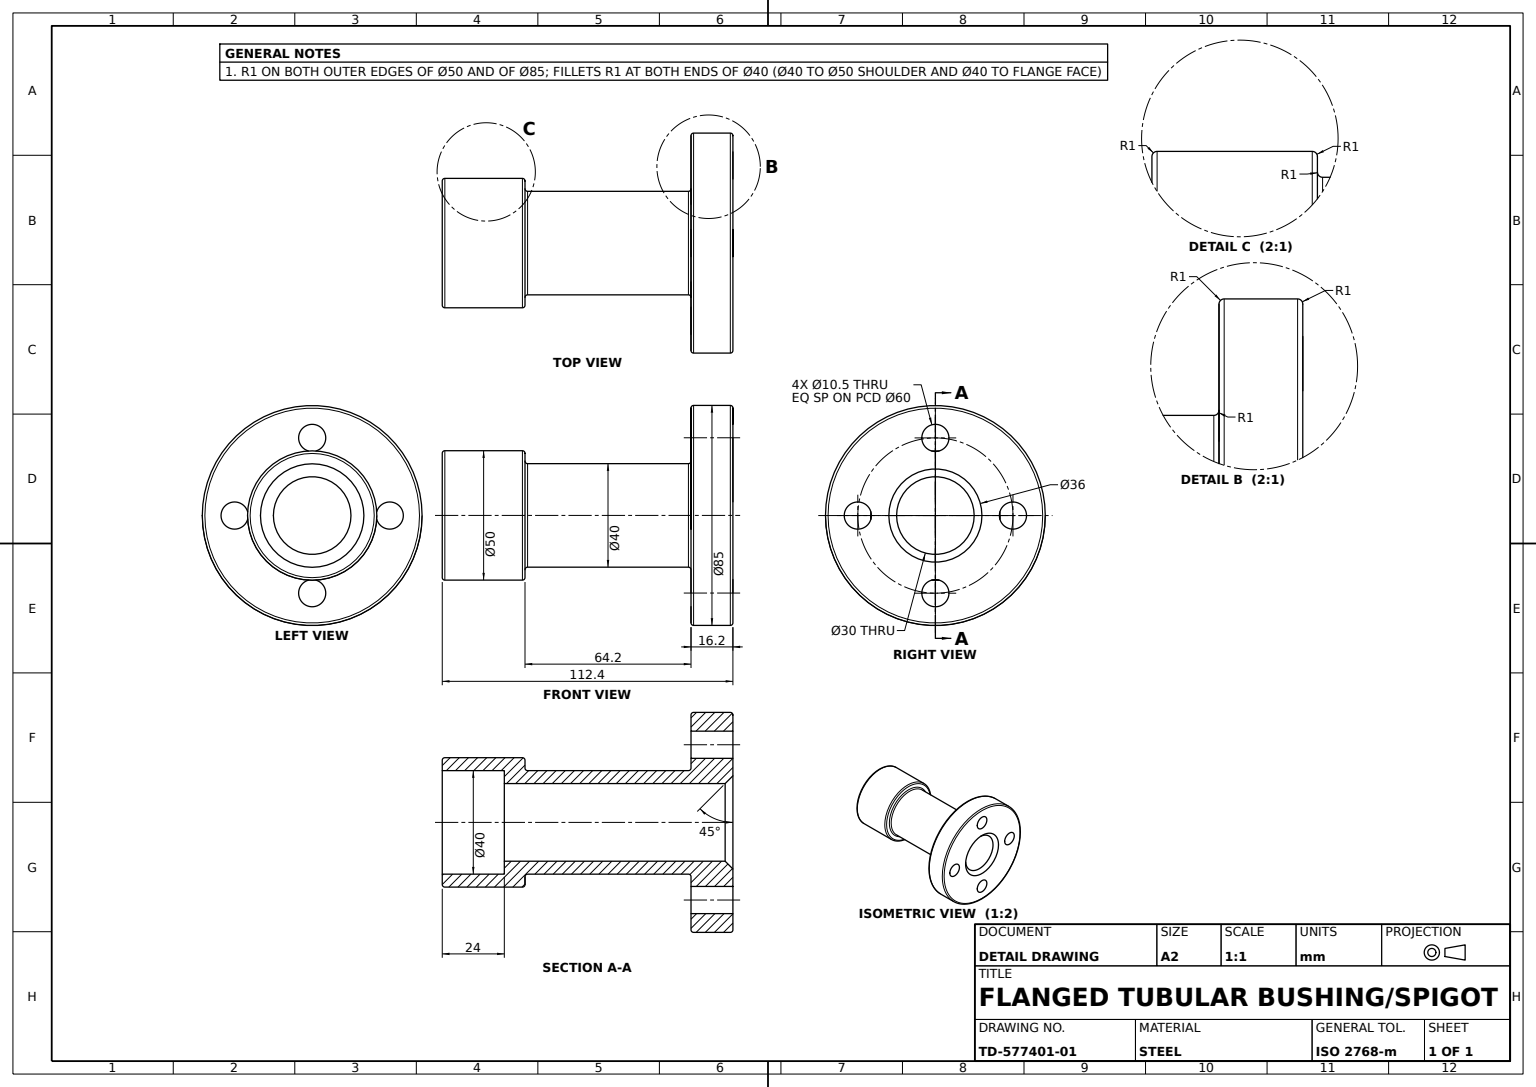
from build123d import *

# Parameters (mm, degrees)
FLANGE_HOLES_SKETCH_R      = 5.25
FLANGE_HOLES_4X_10_5_DEPTH = 39
CHAMFER_3X45_SIZE          = 3
FILLET_R1_R                = 1


with BuildPart() as part:
    # Bush Profile Sketch → Flanged Bush Body (revolve)
    with BuildSketch(Plane(origin=(0, 0, 0), x_dir=(0, 0, -1), z_dir=(1, 0, 0)), mode=Mode.PRIVATE) as flanged_bush_body_sk:
        Polygon((0, 15), (0, 42.5), (-16.2, 42.5), (-16.2, 20), (-80.4, 20), (-80.4, 25), (-112.4, 25), (-112.4, 20), (-88.4, 20), (-88.4, 15), align=None)
    revolve(flanged_bush_body_sk.sketch.rotate(Axis((0, 0, 511.464555616), (0, 0, -1)), 90), axis=Axis((0, 0, 511.464555616), (0, 0, -1)))

    # Flange Holes Sketch → Flange Holes 4xØ10.5 (cut)
    with BuildSketch(Plane(origin=(0, 0, 0), x_dir=(-1, 0, 0), z_dir=(0, 0, -1))):
        with Locations((0, 30)):
            Circle(FLANGE_HOLES_SKETCH_R)
        with Locations((30, 0)):
            Circle(FLANGE_HOLES_SKETCH_R)
        with Locations((0, -30)):
            Circle(FLANGE_HOLES_SKETCH_R)
        with Locations((-30, 0)):
            Circle(FLANGE_HOLES_SKETCH_R)
    extrude(amount=-FLANGE_HOLES_4X_10_5_DEPTH, mode=Mode.SUBTRACT)

    # Chamfer 3x45
    chamfer_3x45_edges = [part.edges().sort_by_distance(p)[0] for p in [
        (-15, 0, 0),
    ]]
    chamfer(chamfer_3x45_edges, length=CHAMFER_3X45_SIZE)

    # Fillet R1
    fillet_r1_edges = [part.edges().sort_by_distance(p)[0] for p in [
        (-20, 0, 80.4),
        (-20, 0, 16.2),
        (-42.5, 0, 16.2),
        (-42.5, 0, 0),
        (-25, 0, 112.4),
        (-25, 0, 80.4),
    ]]
    fillet(fillet_r1_edges, radius=FILLET_R1_R)


solid = part.part
